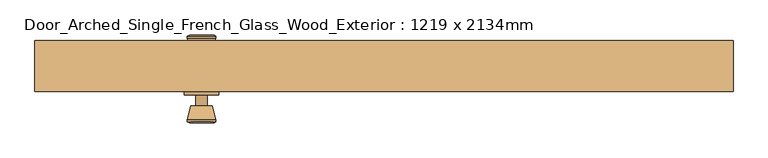
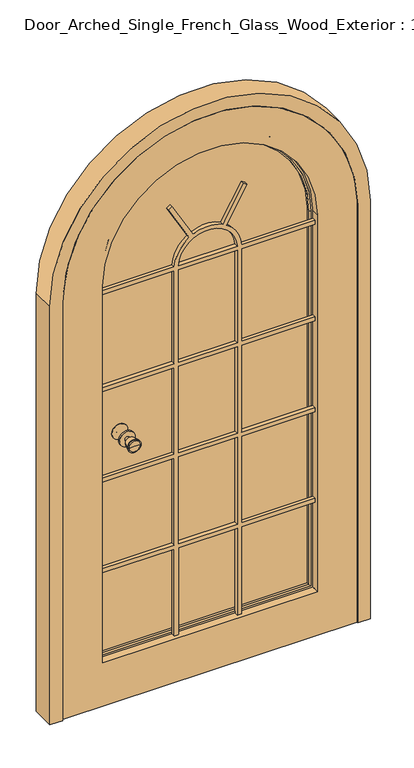
"""IFC4 building model written with IfcOpenShell, lengths in millimetres: door geometry, Door_Arched_Single_French_Glass_Wood_Exterior : 1219 x 2134mm."""

from ifc_helpers import new_model, si_unit, point, frame, frame_2d, origin, place, context, project, spatial, polyline, circle_curve, ellipse_curve, trimmed, segment, composite_curve, outline, extrude, source, transform, mapped, element, save
from ifc_brep_helpers import plane_surface, cylinder_surface, revolved_surface, advanced_brep


def door_arched_single_french_glass_wood_exterior_1219_x_2134mm_7a906126(model_context):
    return source(origin(), model_context, "Body", "SolidModel", [
        advanced_brep(
        [(-318.5, -5.7, 1050.0), (-308.5, -5.7, 1050.0), (-328.5, -5.7, 1050.0), (-298.0241324, -54.7, 1050.0), (-318.5, -54.7, 1050.0), (-338.9758676, -54.7, 1050.0), (-293.5, -52.8721319, 1050.0), (-343.5, -52.8721319, 1050.0), (-293.5, -49.4084537, 1050.0), (-343.5, -49.4084537, 1050.0), (-299.863764, -24.7, 1050.0), (-337.136236, -24.7, 1050.0), (-308.5, -24.7, 1050.0), (-328.5, -24.7, 1050.0)],
        [
            (0, 1),
            (1, 2, circle_curve(frame((-318.5, -5.7, 1050.0), z_axis=(0.0, 1.0, 0.0), x_axis=(-1.0, 0.0, 0.0)), 10.0)),
            (2, 0),
            (2, 1, circle_curve(frame((-318.5, -5.7, 1050.0), z_axis=(0.0, 1.0, 0.0), x_axis=(-1.0, 0.0, 0.0)), 10.0)),
            (3, 4),
            (4, 5),
            (5, 3, circle_curve(frame((-318.5, -54.7, 1050.0), z_axis=(0.0, -1.0, 0.0), x_axis=(-1.0, 0.0, 0.0)), 20.4758676)),
            (3, 5, circle_curve(frame((-318.5, -54.7, 1050.0), z_axis=(0.0, -1.0, 0.0), x_axis=(-1.0, 0.0, 0.0)), 20.4758676)),
            (6, 3),
            (5, 7),
            (7, 6, circle_curve(frame((-318.5, -52.8721319, 1050.0), z_axis=(0.0, -1.0, 0.0), x_axis=(-1.0, 0.0, 0.0)), 25.0)),
            (6, 7, circle_curve(frame((-318.5, -52.8721319, 1050.0), z_axis=(0.0, -1.0, 0.0), x_axis=(-1.0, 0.0, 0.0)), 25.0)),
            (8, 6),
            (7, 9),
            (9, 8, circle_curve(frame((-318.5, -49.4084537, 1050.0), z_axis=(0.0, -1.0, 0.0), x_axis=(-1.0, 0.0, 0.0)), 25.0)),
            (8, 9, circle_curve(frame((-318.5, -49.4084537, 1050.0), z_axis=(0.0, -1.0, 0.0), x_axis=(-1.0, 0.0, 0.0)), 25.0)),
            (10, 8),
            (9, 11),
            (11, 10, circle_curve(frame((-318.5, -24.7, 1050.0), z_axis=(0.0, -1.0, 0.0), x_axis=(-1.0, 0.0, 0.0)), 18.636236)),
            (10, 11, circle_curve(frame((-318.5, -24.7, 1050.0), z_axis=(0.0, -1.0, 0.0), x_axis=(-1.0, 0.0, 0.0)), 18.636236)),
            (12, 10),
            (11, 13),
            (13, 12, circle_curve(frame((-318.5, -24.7, 1050.0), z_axis=(0.0, -1.0, 0.0), x_axis=(-1.0, 0.0, 0.0)), 10.0)),
            (12, 13, circle_curve(frame((-318.5, -24.7, 1050.0), z_axis=(0.0, -1.0, 0.0), x_axis=(-1.0, 0.0, 0.0)), 10.0)),
            (1, 12),
            (13, 2),
        ],
        [
            plane_surface(frame((-318.5, -5.7, 1050.0), z_axis=(0.0, 1.0, 0.0), x_axis=(-1.0, 0.0, 0.0))),
            plane_surface(frame((-318.5, -54.7, 1050.0), z_axis=(0.0, -1.0, 0.0), x_axis=(-1.0, 0.0, 0.0))),
            revolved_surface(polyline([(-338.9758676, -54.7, 1050.0), (-343.5, -52.8721319, 1050.0)]), (-318.5, -5.7, 1050.0), (0.0, 1.0, 0.0)),
            cylinder_surface(frame((-318.5, -5.7, 1050.0), z_axis=(0.0, 1.0, 0.0), x_axis=(-1.0, 0.0, 0.0)), 25.0),
            revolved_surface(polyline([(-343.5, -49.4084537, 1050.0), (-337.136236, -24.7, 1050.0)]), (-318.5, -5.7, 1050.0), (0.0, 1.0, 0.0)),
            plane_surface(frame((-318.5, -24.7, 1050.0), z_axis=(0.0, 1.0, 0.0), x_axis=(-1.0, 0.0, 0.0))),
            cylinder_surface(frame((-318.5, -5.7, 1050.0), z_axis=(0.0, 1.0, 0.0), x_axis=(-1.0, 0.0, 0.0)), 10.0),
        ],
        [
            (0, [[1, 2, 3]]),
            (0, [[-3, 4, -1]]),
            (1, [[5, 6, 7]]),
            (1, [[-6, -5, 8]]),
            (2, [[9, -7, 10, 11]]),
            (2, [[-10, -8, -9, 12]]),
            (3, [[13, -11, 14, 15]]),
            (3, [[-14, -12, -13, 16]]),
            (4, [[17, -15, 18, 19]]),
            (4, [[-18, -16, -17, 20]]),
            (5, [[21, -19, 22, 23]]),
            (5, [[-22, -20, -21, 24]]),
            (6, [[25, -23, 26, -2]]),
            (6, [[-26, -24, -25, -4]]),
        ],
    ),
        extrude(outline(composite_curve([segment(trimmed(circle_curve(frame_2d((1050.0, -318.5)), 30.0), [point((1050.0, -348.5))], [point((1050.0, -288.5))], False, "CARTESIAN"), True, "CONTINUOUS"), segment(trimmed(circle_curve(frame_2d((1050.0, -318.5)), 30.0), [point((1050.0, -288.5))], [point((1050.0, -348.5))], False, "CARTESIAN"), True, "CONTINUOUS")], self_intersect=False)), frame((0.0, -5.7, 0.0), z_axis=(0.0, 1.0, 0.0), x_axis=(0.0, 0.0, 1.0)), (0.0, 0.0, 1.0), 6.0),
        advanced_brep(
        [(-318.5, 50.3, 1050.0), (-328.5, 50.3, 1050.0), (-308.5, 50.3, 1050.0), (-298.0241324, 99.3, 1050.0), (-338.9758676, 99.3, 1050.0), (-318.5, 99.3, 1050.0), (-293.5, 97.4721319, 1050.0), (-343.5, 97.4721319, 1050.0), (-293.5, 94.0084537, 1050.0), (-343.5, 94.0084537, 1050.0), (-299.863764, 69.3, 1050.0), (-337.136236, 69.3, 1050.0), (-308.5, 69.3, 1050.0), (-328.5, 69.3, 1050.0)],
        [
            (0, 1),
            (1, 2, circle_curve(frame((-318.5, 50.3, 1050.0), z_axis=(0.0, -1.0, 0.0), x_axis=(-1.0, 0.0, 0.0)), 10.0)),
            (2, 0),
            (2, 1, circle_curve(frame((-318.5, 50.3, 1050.0), z_axis=(0.0, -1.0, 0.0), x_axis=(-1.0, 0.0, 0.0)), 10.0)),
            (3, 4, circle_curve(frame((-318.5, 99.3, 1050.0), z_axis=(0.0, 1.0, 0.0), x_axis=(-1.0, 0.0, 0.0)), 20.4758676)),
            (4, 5),
            (5, 3),
            (4, 3, circle_curve(frame((-318.5, 99.3, 1050.0), z_axis=(0.0, 1.0, 0.0), x_axis=(-1.0, 0.0, 0.0)), 20.4758676)),
            (6, 7, circle_curve(frame((-318.5, 97.4721319, 1050.0), z_axis=(0.0, 1.0, 0.0), x_axis=(-1.0, 0.0, 0.0)), 25.0)),
            (7, 4),
            (3, 6),
            (7, 6, circle_curve(frame((-318.5, 97.4721319, 1050.0), z_axis=(0.0, 1.0, 0.0), x_axis=(-1.0, 0.0, 0.0)), 25.0)),
            (8, 9, circle_curve(frame((-318.5, 94.0084537, 1050.0), z_axis=(0.0, 1.0, 0.0), x_axis=(-1.0, 0.0, 0.0)), 25.0)),
            (9, 7),
            (6, 8),
            (9, 8, circle_curve(frame((-318.5, 94.0084537, 1050.0), z_axis=(0.0, 1.0, 0.0), x_axis=(-1.0, 0.0, 0.0)), 25.0)),
            (10, 11, circle_curve(frame((-318.5, 69.3, 1050.0), z_axis=(0.0, 1.0, 0.0), x_axis=(-1.0, 0.0, 0.0)), 18.636236)),
            (11, 9),
            (8, 10),
            (11, 10, circle_curve(frame((-318.5, 69.3, 1050.0), z_axis=(0.0, 1.0, 0.0), x_axis=(-1.0, 0.0, 0.0)), 18.636236)),
            (12, 13, circle_curve(frame((-318.5, 69.3, 1050.0), z_axis=(0.0, 1.0, 0.0), x_axis=(-1.0, 0.0, 0.0)), 10.0)),
            (13, 11),
            (10, 12),
            (13, 12, circle_curve(frame((-318.5, 69.3, 1050.0), z_axis=(0.0, 1.0, 0.0), x_axis=(-1.0, 0.0, 0.0)), 10.0)),
            (1, 13),
            (12, 2),
        ],
        [
            plane_surface(frame((-318.5, 50.3, 1050.0), z_axis=(0.0, -1.0, 0.0), x_axis=(-1.0, 0.0, 0.0))),
            plane_surface(frame((-318.5, 99.3, 1050.0), z_axis=(0.0, 1.0, 0.0), x_axis=(-1.0, 0.0, 0.0))),
            revolved_surface(polyline([(-338.9758676, 99.3, 1050.0), (-343.5, 97.4721319, 1050.0)]), (-318.5, 50.3, 1050.0), (0.0, -1.0, 0.0)),
            cylinder_surface(frame((-318.5, 50.3, 1050.0), z_axis=(0.0, -1.0, 0.0), x_axis=(-1.0, 0.0, 0.0)), 25.0),
            revolved_surface(polyline([(-343.5, 94.0084537, 1050.0), (-337.136236, 69.3, 1050.0)]), (-318.5, 50.3, 1050.0), (0.0, -1.0, 0.0)),
            plane_surface(frame((-318.5, 69.3, 1050.0), z_axis=(0.0, -1.0, 0.0), x_axis=(-1.0, 0.0, 0.0))),
            cylinder_surface(frame((-318.5, 50.3, 1050.0), z_axis=(0.0, -1.0, 0.0), x_axis=(-1.0, 0.0, 0.0)), 10.0),
        ],
        [
            (0, [[1, 2, 3]]),
            (0, [[-3, 4, -1]]),
            (1, [[5, 6, 7]]),
            (1, [[8, -7, -6]]),
            (2, [[9, 10, -5, 11]]),
            (2, [[12, -11, -8, -10]]),
            (3, [[13, 14, -9, 15]]),
            (3, [[16, -15, -12, -14]]),
            (4, [[17, 18, -13, 19]]),
            (4, [[20, -19, -16, -18]]),
            (5, [[21, 22, -17, 23]]),
            (5, [[24, -23, -20, -22]]),
            (6, [[-2, 25, -21, 26]]),
            (6, [[-4, -26, -24, -25]]),
        ],
    ),
        extrude(outline(composite_curve([segment(trimmed(circle_curve(frame_2d((1050.0, -318.5)), 30.0), [point((1050.0, -348.5))], [point((1050.0, -288.5))], False, "CARTESIAN"), True, "CONTINUOUS"), segment(trimmed(circle_curve(frame_2d((1050.0, -318.5)), 30.0), [point((1050.0, -288.5))], [point((1050.0, -348.5))], False, "CARTESIAN"), True, "CONTINUOUS")], self_intersect=False)), frame((0.0, 44.3, 0.0), z_axis=(0.0, 1.0, 0.0), x_axis=(0.0, 0.0, 1.0)), (0.0, 0.0, 1.0), 6.0),
        advanced_brep(
        [(539.1, 89.3, 0.0), (609.6, 89.3, 0.0), (609.6, 0.3, 0.0), (561.1, 0.3, 0.0), (561.1, 47.3, 0.0), (539.1, 47.3, 0.0), (539.1, 89.3, 1678.6), (-539.1, 89.3, 1678.6), (-539.1, 89.3, 0.0), (-609.6, 89.3, 0.0), (-609.6, 89.3, 1678.6), (609.6, 89.3, 1678.6), (609.6, 0.3, 1678.6), (-609.6, 0.3, 1678.6), (-609.6, 0.3, 0.0), (-561.1, 0.3, 0.0), (-561.1, 0.3, 1678.6), (561.1, 0.3, 1678.6), (561.1, 47.3, 1678.6), (-561.1, 47.3, 1678.6), (-561.1, 47.3, 0.0), (-539.1, 47.3, 0.0), (-539.1, 47.3, 1678.6), (539.1, 47.3, 1678.6)],
        [
            (0, 1),
            (1, 2),
            (2, 3),
            (3, 4),
            (4, 5),
            (5, 0),
            (0, 6),
            (6, 7, circle_curve(frame((0.0, 89.3, 1678.6), z_axis=(0.0, -1.0, 0.0), x_axis=(1.0, 0.0, 0.0)), 539.1)),
            (7, 8),
            (8, 9),
            (9, 10),
            (10, 11, circle_curve(frame((0.0, 89.3, 1678.6), z_axis=(0.0, 1.0, 0.0), x_axis=(1.0, 0.0, 0.0)), 609.6)),
            (11, 1),
            (11, 12),
            (12, 2),
            (12, 13, circle_curve(frame((0.0, 0.3, 1678.6), z_axis=(0.0, -1.0, 0.0), x_axis=(1.0, 0.0, 0.0)), 609.6)),
            (13, 14),
            (14, 15),
            (15, 16),
            (16, 17, circle_curve(frame((0.0, 0.3, 1678.6), z_axis=(0.0, 1.0, 0.0), x_axis=(1.0, 0.0, 0.0)), 561.1)),
            (17, 3),
            (17, 18),
            (18, 4),
            (18, 19, circle_curve(frame((0.0, 47.3, 1678.6), z_axis=(0.0, -1.0, 0.0), x_axis=(1.0, 0.0, 0.0)), 561.1)),
            (19, 20),
            (20, 21),
            (21, 22),
            (22, 23, circle_curve(frame((0.0, 47.3, 1678.6), z_axis=(0.0, 1.0, 0.0), x_axis=(1.0, 0.0, 0.0)), 539.1)),
            (23, 5),
            (23, 6),
            (7, 22),
            (21, 8),
            (20, 15),
            (14, 9),
            (13, 10),
            (19, 16),
        ],
        [
            plane_surface(frame((603.1, -9.1123976, 0.0), z_axis=(0.0, 0.0, -1.0), x_axis=(1.0, 0.0, 0.0))),
            plane_surface(frame((539.1, 89.3, 0.0), z_axis=(0.0, 1.0, 0.0), x_axis=(0.0, 0.0, 1.0))),
            plane_surface(frame((609.6, 89.3, 0.0), z_axis=(1.0, 0.0, 0.0), x_axis=(0.0, 0.0, 1.0))),
            plane_surface(frame((609.6, 0.3, 0.0), z_axis=(0.0, -1.0, 0.0), x_axis=(0.0, 0.0, 1.0))),
            plane_surface(frame((561.1, 0.3, 0.0), z_axis=(-1.0, 0.0, 0.0), x_axis=(0.0, 0.0, 1.0))),
            plane_surface(frame((561.1, 47.3, 0.0), z_axis=(0.0, -1.0, 0.0), x_axis=(0.0, 0.0, 1.0))),
            plane_surface(frame((539.1, 47.3, 0.0), z_axis=(-1.0, 0.0, 0.0), x_axis=(0.0, 0.0, 1.0))),
            plane_surface(frame((-539.1, 47.3, 1678.6), z_axis=(1.0, 0.0, 0.0), x_axis=(0.0, 0.0, -1.0))),
            plane_surface(frame((-603.1, -9.1123976, 0.0), z_axis=(0.0, 0.0, -1.0), x_axis=(-1.0, 0.0, 0.0))),
            plane_surface(frame((-609.6, 89.3, 1678.6), z_axis=(-1.0, 0.0, 0.0), x_axis=(0.0, 0.0, -1.0))),
            plane_surface(frame((-561.1, 0.3, 1678.6), z_axis=(1.0, 0.0, 0.0), x_axis=(0.0, 0.0, -1.0))),
            cylinder_surface(frame((0.0, 89.3, 1678.6), z_axis=(0.0, -1.0, 0.0), x_axis=(1.0, 0.0, 0.0)), 609.6),
            revolved_surface(polyline([(561.1, 0.29999999999999716, 1678.6), (561.1, 47.3, 1678.6)]), (0.0, 89.3, 1678.6), (0.0, -1.0, 0.0)),
            revolved_surface(polyline([(539.1, 47.3, 1678.6), (539.1, 89.3, 1678.6)]), (0.0, 89.3, 1678.6), (0.0, -1.0, 0.0)),
        ],
        [
            (0, [[1, 2, 3, 4, 5, 6]]),
            (1, [[-1, 7, 8, 9, 10, 11, 12, 13]]),
            (2, [[-2, -13, 14, 15]]),
            (3, [[-3, -15, 16, 17, 18, 19, 20, 21]]),
            (4, [[-4, -21, 22, 23]]),
            (5, [[-5, -23, 24, 25, 26, 27, 28, 29]]),
            (6, [[-6, -29, 30, -7]]),
            (7, [[31, -27, 32, -9]]),
            (8, [[-32, -26, 33, -18, 34, -10]]),
            (9, [[35, -11, -34, -17]]),
            (10, [[36, -19, -33, -25]]),
            (11, [[-16, -14, -12, -35]]),
            (12, [[-24, -22, -20, -36]]),
            (13, [[-8, -30, -28, -31]]),
        ],
    ),
        extrude(outline(composite_curve([segment(trimmed(circle_curve(frame_2d((1692.1, 0.0)), 253.5), [point((1896.740356, 149.6147543))], [point((1905.7961472, 136.3679092))], False, "CARTESIAN"), True, "CONTINUOUS"), segment(polyline([(1905.7961472, 136.3679092), (1768.2345335, 56.9466745)]), True, "CONTINUOUS"), segment(trimmed(circle_curve(frame_2d((1653.6, 0.0)), 128.0), [point((1768.2345335, 56.9466745))], [point((1768.2345335, -56.9466745))], False, "CARTESIAN"), True, "CONTINUOUS"), segment(polyline([(1768.2345335, -56.9466745), (1905.7961472, -136.3679092)]), True, "CONTINUOUS"), segment(trimmed(circle_curve(frame_2d((1692.1, 0.0)), 253.5), [point((1905.7961472, -136.3679092))], [point((1896.740356, -149.6147543))], False, "CARTESIAN"), True, "CONTINUOUS"), segment(polyline([(1896.740356, -149.6147543), (1760.2345335, -70.8030809)]), True, "CONTINUOUS"), segment(trimmed(circle_curve(frame_2d((1653.6, 0.0)), 128.0), [point((1760.2345335, -70.8030809))], [point((1661.6, -127.7497554))], False, "CARTESIAN"), True, "CONTINUOUS"), segment(polyline([(1661.6, -127.7497554), (1661.6, -408.1), (1645.6, -408.1), (1645.6, -128.0), (1273.5, -128.0), (1273.5, -408.1), (1257.5, -408.1), (1257.5, -128.0), (909.0, -128.0), (909.0, -408.1), (893.0, -408.1), (893.0, -128.0), (544.5, -128.0), (544.5, -408.1), (528.5, -408.1), (528.5, -128.0), (179.0, -128.0), (179.0, -112.0), (528.5, -112.0), (528.5, 112.0), (179.0, 112.0), (179.0, 128.0), (528.5, 128.0), (528.5, 408.1), (544.5, 408.1), (544.5, 128.0), (893.0, 128.0), (893.0, 408.1), (909.0, 408.1), (909.0, 128.0), (1257.5, 128.0), (1257.5, 408.1), (1273.5, 408.1), (1273.5, 128.0), (1645.6, 128.0), (1645.6, 408.1), (1661.6, 408.1), (1661.6, 127.7497554)]), True, "CONTINUOUS"), segment(trimmed(circle_curve(frame_2d((1653.6, 0.0)), 128.0), [point((1661.6, 127.7497554))], [point((1760.2345335, 70.8030809))], False, "CARTESIAN"), True, "CONTINUOUS"), segment(polyline([(1760.2345335, 70.8030809), (1896.740356, 149.6147543)]), True, "CONTINUOUS")], self_intersect=False), holes=[polyline([(893.0, -112.0), (893.0, 112.0), (544.5, 112.0), (544.5, -112.0), (893.0, -112.0)]), polyline([(1257.5, 112.0), (909.0, 112.0), (909.0, -112.0), (1257.5, -112.0), (1257.5, 112.0)]), composite_curve([segment(trimmed(circle_curve(frame_2d((1653.6, 0.0)), 112.0), [point((1661.6, -111.7139204))], [point((1661.6, 111.7139204))], True, "CARTESIAN"), True, "CONTINUOUS"), segment(polyline([(1661.6, 111.7139204), (1661.6, -111.7139204)]), True, "CONTINUOUS")], self_intersect=False), polyline([(1645.6, -112.0), (1645.6, 112.0), (1273.5, 112.0), (1273.5, -112.0), (1645.6, -112.0)])]), frame((0.0, 15.1515468, 0.0), z_axis=(0.0, 1.0, 0.0), x_axis=(0.0, 0.0, 1.0)), (0.0, 0.0, 1.0), 14.5359085),
        extrude(outline(composite_curve([segment(polyline([(4.0, 558.1), (1727.8950302, 558.1)]), True, "CONTINUOUS"), segment(trimmed(circle_curve(frame_2d((1678.6, 0.0)), 560.2727996), [point((1727.8950302, 558.1))], [point((1715.9714663, -559.0250294))], False, "CARTESIAN"), True, "CONTINUOUS"), segment(polyline([(1715.9714663, -559.0250294), (4.0, -559.0250294), (4.0, 558.1)]), True, "CONTINUOUS")], self_intersect=False), holes=[composite_curve([segment(polyline([(179.0, -408.1), (1692.1, -408.1)]), True, "CONTINUOUS"), segment(trimmed(circle_curve(frame_2d((1692.1, 0.0)), 408.1), [point((1692.1, -408.1))], [point((1692.1, 408.1))], True, "CARTESIAN"), True, "CONTINUOUS"), segment(polyline([(1692.1, 408.1), (179.0, 408.1), (179.0, -408.1)]), True, "CONTINUOUS")], self_intersect=False)]), frame((0.0, 0.3, 0.0), z_axis=(0.0, 1.0, 0.0), x_axis=(0.0, 0.0, 1.0)), (0.0, 0.0, 1.0), 44.0),
        extrude(outline(composite_curve([segment(polyline([(179.0, -408.1), (179.0, 408.1), (1692.1, 408.1)]), True, "CONTINUOUS"), segment(trimmed(circle_curve(frame_2d((1692.1, 0.0)), 408.1), [point((1692.1, 408.1))], [point((1692.1, -408.1))], False, "CARTESIAN"), True, "CONTINUOUS"), segment(polyline([(1692.1, -408.1), (179.0, -408.1)]), True, "CONTINUOUS")], self_intersect=False)), frame((0.0, 46.0, 0.0), z_axis=(0.0, 1.0, 0.0), x_axis=(0.0, 0.0, 1.0)), (0.0, 0.0, 1.0), 24.0),
        advanced_brep(
        [(-416.1, 84.0, 171.0), (-416.1, 80.0, 171.0), (-416.1, 80.0, 1692.1), (-416.1, 84.0, 1692.1), (-414.1, 86.0, 173.0), (-414.1, 86.0, 1692.1), (-396.1, 81.0, 191.0), (-401.1, 86.0, 186.0), (-401.1, 86.0, 1692.1), (-396.1, 81.0, 1692.1), (-396.1, 70.0, 191.0), (-396.1, 70.0, 1692.1), (-408.1, 80.0, 179.0), (-408.1, 70.0, 179.0), (-408.1, 70.0, 1692.1), (-408.1, 80.0, 1692.1), (416.1, 84.0, 1692.1), (416.1, 80.0, 1692.1), (414.1, 86.0, 1692.1), (414.1, 86.0, 173.0), (401.1, 86.0, 1692.1), (401.1, 86.0, 186.0), (396.1, 81.0, 1692.1), (396.1, 70.0, 1692.1), (408.1, 70.0, 1692.1), (408.1, 70.0, 179.0), (396.1, 70.0, 191.0), (408.1, 80.0, 1692.1), (416.1, 80.0, 171.0), (408.1, 80.0, 179.0), (416.1, 84.0, 171.0), (396.1, 81.0, 191.0)],
        [
            (0, 1),
            (1, 2),
            (2, 3),
            (3, 0),
            (4, 0, ellipse_curve(frame((-414.1, 84.0, 173.0), z_axis=(-0.7071067811865475, 0.0, 0.7071067811865475), x_axis=(-0.7071067811865474, 0.0, -0.7071067811865476)), 2.8284271, 2.0)),
            (3, 5, circle_curve(frame((-414.1, 84.0, 1692.1), z_axis=(0.0, 0.0, -1.0), x_axis=(-1.0, 0.0, 0.0)), 2.0)),
            (5, 4),
            (6, 7, ellipse_curve(frame((-401.1, 81.0, 186.0), z_axis=(-0.7071067811865475, 0.0, 0.7071067811865475), x_axis=(-0.7071067811865474, 0.0, -0.7071067811865476)), 7.0710678, 5.0)),
            (7, 8),
            (8, 9, circle_curve(frame((-401.1, 81.0, 1692.1), z_axis=(0.0, 0.0, -1.0), x_axis=(-1.0, 0.0, 0.0)), 5.0)),
            (9, 6),
            (10, 6),
            (9, 11),
            (11, 10),
            (12, 13),
            (13, 14),
            (14, 15),
            (15, 12),
            (16, 3, circle_curve(frame((0.0, 84.0, 1692.1), z_axis=(0.0, -1.0, 0.0), x_axis=(-1.0, 0.0, 0.0)), 416.1)),
            (2, 17, circle_curve(frame((0.0, 80.0, 1692.1), z_axis=(0.0, 1.0, 0.0), x_axis=(-1.0, 0.0, 0.0)), 416.1)),
            (17, 16),
            (18, 5, circle_curve(frame((0.0, 86.0, 1692.1), z_axis=(0.0, -1.0, 0.0), x_axis=(-1.0, 0.0, 0.0)), 414.1)),
            (16, 18, circle_curve(frame((414.1, 84.0, 1692.1), z_axis=(0.0, 0.0, 1.0), x_axis=(1.0, 0.0, 0.0)), 2.0)),
            (18, 19),
            (19, 4),
            (20, 8, circle_curve(frame((0.0, 86.0, 1692.1), z_axis=(0.0, -1.0, 0.0), x_axis=(-1.0, 0.0, 0.0)), 401.1)),
            (7, 21),
            (21, 20),
            (22, 9, circle_curve(frame((0.0, 81.0, 1692.1), z_axis=(0.0, -1.0, 0.0), x_axis=(-1.0, 0.0, 0.0)), 396.1)),
            (20, 22, circle_curve(frame((401.1, 81.0, 1692.1), z_axis=(0.0, 0.0, 1.0), x_axis=(1.0, 0.0, 0.0)), 5.0)),
            (23, 11, circle_curve(frame((0.0, 70.0, 1692.1), z_axis=(0.0, -1.0, 0.0), x_axis=(-1.0, 0.0, 0.0)), 396.1)),
            (22, 23),
            (24, 14, circle_curve(frame((0.0, 70.0, 1692.1), z_axis=(0.0, -1.0, 0.0), x_axis=(-1.0, 0.0, 0.0)), 408.1)),
            (13, 25),
            (25, 24),
            (23, 26),
            (26, 10),
            (27, 15, circle_curve(frame((0.0, 80.0, 1692.1), z_axis=(0.0, -1.0, 0.0), x_axis=(-1.0, 0.0, 0.0)), 408.1)),
            (24, 27),
            (1, 28),
            (28, 17),
            (27, 29),
            (29, 12),
            (28, 30),
            (30, 16),
            (30, 19, ellipse_curve(frame((414.1, 84.0, 173.0), z_axis=(0.7071067811865475, 0.0, 0.7071067811865475), x_axis=(-0.7071067811865474, 0.0, 0.7071067811865476)), 2.8284271, 2.0)),
            (21, 31, ellipse_curve(frame((401.1, 81.0, 186.0), z_axis=(0.7071067811865475, 0.0, 0.7071067811865475), x_axis=(-0.7071067811865474, 0.0, 0.7071067811865476)), 7.0710678, 5.0)),
            (31, 22),
            (31, 26),
            (25, 29),
            (0, 30),
            (6, 31),
        ],
        [
            plane_surface(frame((-416.1, 80.0, 171.0), z_axis=(-1.0, 0.0, 0.0), x_axis=(0.0, 0.0, 1.0))),
            cylinder_surface(frame((-414.1, 84.0, 179.0), z_axis=(0.0, 0.0, -1.0), x_axis=(-1.0, 0.0, 0.0)), 2.0),
            cylinder_surface(frame((-401.1, 81.0, 179.0), z_axis=(0.0, 0.0, -1.0), x_axis=(-1.0, 0.0, 0.0)), 5.0),
            plane_surface(frame((-396.1, 81.0, 191.0), z_axis=(1.0, 0.0, 0.0), x_axis=(0.0, 0.0, 1.0))),
            plane_surface(frame((-408.1, 70.0, 179.0), z_axis=(-1.0, 0.0, 0.0), x_axis=(0.0, 0.0, 1.0))),
            cylinder_surface(frame((0.0, 80.0, 1692.1), z_axis=(0.0, 1.0, 0.0), x_axis=(-1.0, 0.0, 0.0)), 416.1),
            revolved_surface(trimmed(ellipse_curve(frame((-414.1, 84.0, 1692.1), z_axis=(0.0, 0.0, -1.0), x_axis=(-1.0, 0.0, 0.0)), 2.0, 2.0), [point((-416.1, 84.0, 1692.1))], [point((-414.1, 86.0, 1692.1))], True, "CARTESIAN"), (0.0, 80.0, 1692.1), (0.0, 1.0, 0.0)),
            plane_surface(frame((0.0, 86.0, 1692.1), z_axis=(0.0, 1.0, 0.0), x_axis=(-1.0, 0.0, 0.0))),
            revolved_surface(trimmed(ellipse_curve(frame((-401.1, 81.0, 1692.1), z_axis=(0.0, 0.0, -1.0), x_axis=(-1.0, 0.0, 0.0)), 5.0, 5.0), [point((-401.1, 86.0, 1692.1))], [point((-396.1, 81.0, 1692.1))], True, "CARTESIAN"), (0.0, 80.0, 1692.1), (0.0, 1.0, 0.0)),
            revolved_surface(polyline([(-396.1, 81.0, 1692.1), (-396.1, 70.0, 1692.1)]), (0.0, 80.0, 1692.1), (0.0, 1.0, 0.0)),
            plane_surface(frame((0.0, 70.0, 1692.1), z_axis=(0.0, -1.0, 0.0), x_axis=(-1.0, 0.0, 0.0))),
            cylinder_surface(frame((0.0, 80.0, 1692.1), z_axis=(0.0, 1.0, 0.0), x_axis=(-1.0, 0.0, 0.0)), 408.1),
            plane_surface(frame((0.0, 80.0, 1692.1), z_axis=(0.0, -1.0, 0.0), x_axis=(-1.0, 0.0, 0.0))),
            plane_surface(frame((416.1, 80.0, 1692.1), z_axis=(1.0, 0.0, 0.0), x_axis=(0.0, 0.0, -1.0))),
            cylinder_surface(frame((414.1, 84.0, 1692.1), z_axis=(0.0, 0.0, 1.0), x_axis=(1.0, 0.0, 0.0)), 2.0),
            cylinder_surface(frame((401.1, 81.0, 1692.1), z_axis=(0.0, 0.0, 1.0), x_axis=(1.0, 0.0, 0.0)), 5.0),
            plane_surface(frame((396.1, 81.0, 1692.1), z_axis=(-1.0, 0.0, 0.0), x_axis=(0.0, 0.0, -1.0))),
            plane_surface(frame((408.1, 70.0, 1692.1), z_axis=(1.0, 0.0, 0.0), x_axis=(0.0, 0.0, -1.0))),
            plane_surface(frame((416.1, 80.0, 171.0), z_axis=(0.0, 0.0, -1.0), x_axis=(-1.0, 0.0, 0.0))),
            cylinder_surface(frame((408.1, 84.0, 173.0), z_axis=(1.0, 0.0, 0.0), x_axis=(0.0, 0.0, -1.0)), 2.0),
            cylinder_surface(frame((408.1, 81.0, 186.0), z_axis=(1.0, 0.0, 0.0), x_axis=(0.0, 0.0, -1.0)), 5.0),
            plane_surface(frame((396.1, 81.0, 191.0), z_axis=(0.0, 0.0, 1.0), x_axis=(-1.0, 0.0, 0.0))),
            plane_surface(frame((408.1, 70.0, 179.0), z_axis=(0.0, 0.0, -1.0), x_axis=(-1.0, 0.0, 0.0))),
        ],
        [
            (0, [[1, 2, 3, 4]]),
            (1, [[5, -4, 6, 7]]),
            (2, [[8, 9, 10, 11]]),
            (3, [[12, -11, 13, 14]]),
            (4, [[15, 16, 17, 18]]),
            (5, [[19, -3, 20, 21]]),
            (6, [[22, -6, -19, 23]]),
            (7, [[24, 25, -7, -22], [26, -9, 27, 28]]),
            (8, [[29, -10, -26, 30]]),
            (9, [[31, -13, -29, 32]]),
            (10, [[33, -16, 34, 35], [36, 37, -14, -31]]),
            (11, [[38, -17, -33, 39]]),
            (12, [[-20, -2, 40, 41], [42, 43, -18, -38]]),
            (13, [[-21, -41, 44, 45]]),
            (14, [[-23, -45, 46, -24]]),
            (15, [[-30, -28, 47, 48]]),
            (16, [[-32, -48, 49, -36]]),
            (17, [[-39, -35, 50, -42]]),
            (18, [[-44, -40, -1, 51]]),
            (19, [[-46, -51, -5, -25]]),
            (20, [[-47, -27, -8, 52]]),
            (21, [[-49, -52, -12, -37]]),
            (22, [[-50, -34, -15, -43]]),
        ],
    ),
        advanced_brep(
        [(416.1, 32.0, 171.0), (416.1, 36.0, 171.0), (416.1, 36.0, 1692.1), (416.1, 32.0, 1692.1), (414.1, 30.0, 173.0), (414.1, 30.0, 1692.1), (396.1, 35.0, 191.0), (401.1, 30.0, 186.0), (401.1, 30.0, 1692.1), (396.1, 35.0, 1692.1), (396.1, 46.0, 191.0), (396.1, 46.0, 1692.1), (408.1, 36.0, 179.0), (408.1, 46.0, 179.0), (408.1, 46.0, 1692.1), (408.1, 36.0, 1692.1), (-416.1, 32.0, 1692.1), (-416.1, 36.0, 1692.1), (-414.1, 30.0, 1692.1), (-414.1, 30.0, 173.0), (-401.1, 30.0, 1692.1), (-401.1, 30.0, 186.0), (-396.1, 35.0, 1692.1), (-396.1, 46.0, 1692.1), (-408.1, 46.0, 1692.1), (-408.1, 46.0, 179.0), (-396.1, 46.0, 191.0), (-408.1, 36.0, 1692.1), (-416.1, 36.0, 171.0), (-408.1, 36.0, 179.0), (-416.1, 32.0, 171.0), (-396.1, 35.0, 191.0)],
        [
            (0, 1),
            (1, 2),
            (2, 3),
            (3, 0),
            (4, 0, ellipse_curve(frame((414.1, 32.0, 173.0), z_axis=(0.7071067811865475, 0.0, 0.7071067811865475), x_axis=(0.7071067811865474, 0.0, -0.7071067811865476)), 2.8284271, 2.0)),
            (3, 5, circle_curve(frame((414.1, 32.0, 1692.1), z_axis=(0.0, 0.0, -1.0), x_axis=(1.0, 0.0, 0.0)), 2.0)),
            (5, 4),
            (6, 7, ellipse_curve(frame((401.1, 35.0, 186.0), z_axis=(0.7071067811865475, 0.0, 0.7071067811865475), x_axis=(0.7071067811865474, 0.0, -0.7071067811865476)), 7.0710678, 5.0)),
            (7, 8),
            (8, 9, circle_curve(frame((401.1, 35.0, 1692.1), z_axis=(0.0, 0.0, -1.0), x_axis=(1.0, 0.0, 0.0)), 5.0)),
            (9, 6),
            (10, 6),
            (9, 11),
            (11, 10),
            (12, 13),
            (13, 14),
            (14, 15),
            (15, 12),
            (16, 3, circle_curve(frame((0.0, 32.0, 1692.1), z_axis=(0.0, 1.0, 0.0), x_axis=(1.0, 0.0, 0.0)), 416.1)),
            (2, 17, circle_curve(frame((0.0, 36.0, 1692.1), z_axis=(0.0, -1.0, 0.0), x_axis=(1.0, 0.0, 0.0)), 416.1)),
            (17, 16),
            (18, 5, circle_curve(frame((0.0, 30.0, 1692.1), z_axis=(0.0, 1.0, 0.0), x_axis=(1.0, 0.0, 0.0)), 414.1)),
            (16, 18, circle_curve(frame((-414.1, 32.0, 1692.1), z_axis=(0.0, 0.0, 1.0), x_axis=(-1.0, 0.0, 0.0)), 2.0)),
            (18, 19),
            (19, 4),
            (20, 8, circle_curve(frame((0.0, 30.0, 1692.1), z_axis=(0.0, 1.0, 0.0), x_axis=(1.0, 0.0, 0.0)), 401.1)),
            (7, 21),
            (21, 20),
            (22, 9, circle_curve(frame((0.0, 35.0, 1692.1), z_axis=(0.0, 1.0, 0.0), x_axis=(1.0, 0.0, 0.0)), 396.1)),
            (20, 22, circle_curve(frame((-401.1, 35.0, 1692.1), z_axis=(0.0, 0.0, 1.0), x_axis=(-1.0, 0.0, 0.0)), 5.0)),
            (23, 11, circle_curve(frame((0.0, 46.0, 1692.1), z_axis=(0.0, 1.0, 0.0), x_axis=(1.0, 0.0, 0.0)), 396.1)),
            (22, 23),
            (24, 14, circle_curve(frame((0.0, 46.0, 1692.1), z_axis=(0.0, 1.0, 0.0), x_axis=(1.0, 0.0, 0.0)), 408.1)),
            (13, 25),
            (25, 24),
            (23, 26),
            (26, 10),
            (27, 15, circle_curve(frame((0.0, 36.0, 1692.1), z_axis=(0.0, 1.0, 0.0), x_axis=(1.0, 0.0, 0.0)), 408.1)),
            (24, 27),
            (1, 28),
            (28, 17),
            (27, 29),
            (29, 12),
            (28, 30),
            (30, 16),
            (30, 19, ellipse_curve(frame((-414.1, 32.0, 173.0), z_axis=(-0.7071067811865475, 0.0, 0.7071067811865475), x_axis=(0.7071067811865474, 0.0, 0.7071067811865476)), 2.8284271, 2.0)),
            (21, 31, ellipse_curve(frame((-401.1, 35.0, 186.0), z_axis=(-0.7071067811865475, 0.0, 0.7071067811865475), x_axis=(0.7071067811865474, 0.0, 0.7071067811865476)), 7.0710678, 5.0)),
            (31, 22),
            (31, 26),
            (25, 29),
            (0, 30),
            (6, 31),
        ],
        [
            plane_surface(frame((416.1, 36.0, 171.0), z_axis=(1.0, 0.0, 0.0), x_axis=(0.0, 0.0, 1.0))),
            cylinder_surface(frame((414.1, 32.0, 179.0), z_axis=(0.0, 0.0, -1.0), x_axis=(1.0, 0.0, 0.0)), 2.0),
            cylinder_surface(frame((401.1, 35.0, 179.0), z_axis=(0.0, 0.0, -1.0), x_axis=(1.0, 0.0, 0.0)), 5.0),
            plane_surface(frame((396.1, 35.0, 191.0), z_axis=(-1.0, 0.0, 0.0), x_axis=(0.0, 0.0, 1.0))),
            plane_surface(frame((408.1, 46.0, 179.0), z_axis=(1.0, 0.0, 0.0), x_axis=(0.0, 0.0, 1.0))),
            cylinder_surface(frame((0.0, 36.0, 1692.1), z_axis=(0.0, -1.0, 0.0), x_axis=(1.0, 0.0, 0.0)), 416.1),
            revolved_surface(trimmed(ellipse_curve(frame((414.1, 32.0, 1692.1), z_axis=(0.0, 0.0, -1.0), x_axis=(1.0, 0.0, 0.0)), 2.0, 2.0), [point((416.1, 32.0, 1692.1))], [point((414.1, 30.0, 1692.1))], True, "CARTESIAN"), (0.0, 36.0, 1692.1), (0.0, -1.0, 0.0)),
            plane_surface(frame((0.0, 30.0, 1692.1), z_axis=(0.0, -1.0, 0.0), x_axis=(1.0, 0.0, 0.0))),
            revolved_surface(trimmed(ellipse_curve(frame((401.1, 35.0, 1692.1), z_axis=(0.0, 0.0, -1.0), x_axis=(1.0, 0.0, 0.0)), 5.0, 5.0), [point((401.1, 30.0, 1692.1))], [point((396.1, 35.0, 1692.1))], True, "CARTESIAN"), (0.0, 36.0, 1692.1), (0.0, -1.0, 0.0)),
            revolved_surface(polyline([(396.1, 35.0, 1692.1), (396.1, 46.0, 1692.1)]), (0.0, 36.0, 1692.1), (0.0, -1.0, 0.0)),
            plane_surface(frame((0.0, 46.0, 1692.1), z_axis=(0.0, 1.0, 0.0), x_axis=(1.0, 0.0, 0.0))),
            cylinder_surface(frame((0.0, 36.0, 1692.1), z_axis=(0.0, -1.0, 0.0), x_axis=(1.0, 0.0, 0.0)), 408.1),
            plane_surface(frame((0.0, 36.0, 1692.1), z_axis=(0.0, 1.0, 0.0), x_axis=(1.0, 0.0, 0.0))),
            plane_surface(frame((-416.1, 36.0, 1692.1), z_axis=(-1.0, 0.0, 0.0), x_axis=(0.0, 0.0, -1.0))),
            cylinder_surface(frame((-414.1, 32.0, 1692.1), z_axis=(0.0, 0.0, 1.0), x_axis=(-1.0, 0.0, 0.0)), 2.0),
            cylinder_surface(frame((-401.1, 35.0, 1692.1), z_axis=(0.0, 0.0, 1.0), x_axis=(-1.0, 0.0, 0.0)), 5.0),
            plane_surface(frame((-396.1, 35.0, 1692.1), z_axis=(1.0, 0.0, 0.0), x_axis=(0.0, 0.0, -1.0))),
            plane_surface(frame((-408.1, 46.0, 1692.1), z_axis=(-1.0, 0.0, 0.0), x_axis=(0.0, 0.0, -1.0))),
            plane_surface(frame((-416.1, 36.0, 171.0), z_axis=(0.0, 0.0, -1.0), x_axis=(1.0, 0.0, 0.0))),
            cylinder_surface(frame((-408.1, 32.0, 173.0), z_axis=(-1.0, 0.0, 0.0), x_axis=(0.0, 0.0, -1.0)), 2.0),
            cylinder_surface(frame((-408.1, 35.0, 186.0), z_axis=(-1.0, 0.0, 0.0), x_axis=(0.0, 0.0, -1.0)), 5.0),
            plane_surface(frame((-396.1, 35.0, 191.0), z_axis=(0.0, 0.0, 1.0), x_axis=(1.0, 0.0, 0.0))),
            plane_surface(frame((-408.1, 46.0, 179.0), z_axis=(0.0, 0.0, -1.0), x_axis=(1.0, 0.0, 0.0))),
        ],
        [
            (0, [[1, 2, 3, 4]]),
            (1, [[5, -4, 6, 7]]),
            (2, [[8, 9, 10, 11]]),
            (3, [[12, -11, 13, 14]]),
            (4, [[15, 16, 17, 18]]),
            (5, [[19, -3, 20, 21]]),
            (6, [[22, -6, -19, 23]]),
            (7, [[24, 25, -7, -22], [26, -9, 27, 28]]),
            (8, [[29, -10, -26, 30]]),
            (9, [[31, -13, -29, 32]]),
            (10, [[33, -16, 34, 35], [36, 37, -14, -31]]),
            (11, [[38, -17, -33, 39]]),
            (12, [[-20, -2, 40, 41], [42, 43, -18, -38]]),
            (13, [[-21, -41, 44, 45]]),
            (14, [[-23, -45, 46, -24]]),
            (15, [[-30, -28, 47, 48]]),
            (16, [[-32, -48, 49, -36]]),
            (17, [[-39, -35, 50, -42]]),
            (18, [[-44, -40, -1, 51]]),
            (19, [[-46, -51, -5, -25]]),
            (20, [[-47, -27, -8, 52]]),
            (21, [[-49, -52, -12, -37]]),
            (22, [[-50, -34, -15, -43]]),
        ],
    ),
    ])


if __name__ == "__main__":
    model = new_model("IFC4")
    model_context = context("Model", 3, world=origin())
    ifc_project = project(units=[si_unit("LENGTHUNIT", "METRE", prefix="MILLI")], contexts=[model_context])
    site = spatial("IfcSite", under=ifc_project)
    building = spatial("IfcBuilding", under=site)
    placement = place(None, origin())
    door_arched_single_french_glass_wood_exterior_1219_x_2134mm_shape = door_arched_single_french_glass_wood_exterior_1219_x_2134mm_7a906126(model_context)
    element("IfcDoor", 1, ObjectType="Door_Arched_Single_French_Glass_Wood_Exterior : 1219 x 2134mm", at=placement, inside=building, context=model_context, shape_type="MappedRepresentation", body=[
        mapped(door_arched_single_french_glass_wood_exterior_1219_x_2134mm_shape, transform((0.0, 0.0, 0.0), x_axis=(1.0, 0.0, 0.0), y_axis=(0.0, 1.0, 0.0), z_axis=(0.0, 0.0, 1.0))),
    ])
    save(model, "model.ifc")

# Revit data of these elements
# Type "Door_Arched_Single_French_Glass_Wood_Exterior : 1219 x 2134mm"
#   Type Mark = "12"
#   Type Comments = "External Single"
#   Operation = "SingleSwingRight"
#   Keynote = "L20"
#   Analytic Construction = "<None>"
#   Wrap Layers (Int) from Ext = 0' - 6.98819"
#   Wrap Layers (Ext) from Ext = 0' - 4.03543"
#   Thickness = 0' - 1.73228"
#   Stile Shutting = 0' - 5.90551"
#   Stile - Top Rail = 0' - 5.90551"
#   Stile - Hanging = 0' - 5.90551"
#   Stile - Bottom Rail = 0' - 6.88976"
#   Rough Width = 4' - 0"
#   Rough Height = 7' - 0"
#   O/A Frame Width = 0' - 2.51969"
#   Handle Z Distance = 3' - 5.33858"
#   Glazing Thickness = 0' - 0.94488"
#   Glazing Bar Thickness = 0' - 0.7874"
#   FrameWidth = 0' - 1.65354"
#   FrameOffset - External = 0' - 0.98425"
#   FrameDepth = 0' - 3.50394"
#   Door Panel Width = 3' - 7.94488"
#   Handle X Distance = 0' - 2.95276"
#   Height = 7' - 0"
#   Structural Tolerance = 0' - 0.25591"
#   Tolerance = 0' - 0.11811"
#   Undercut = 0' - 0.15748"
#   Width = 4' - 0"
#   Door Panel Thickness = 0' - 1.73228"
#   Door Panel Height = 6' - 9.81496"
#   Cavity Closer Width = 0' - 1.9685"
#   Cavity Closer Offset from Ext = 0' - 4.03543"
#   Cavity Closer Depth = 0' - 3.34646"
#   Vis - Ironmongery = yes
#   Vis - Cavity Closers = yes
#   Define Thermal Properties by = 1
#   Material Glass = Door - Glazing
#   Handle Style = element 451349
#   Material Door = Door - Panel
#   Material Frame = BROWN
#   Material Ironmongery = Door - Handle
#   Function = (empty or 0)
#   Wall Closure = (empty or 0)
#   Assembly Code = ""
# Element 1 (IfcDoor, "Door_Arched_Single_French_Glass_Wood_Exterior : 1219 x 2134mm")
#   Materials on its faces: "Door - Panel", "Door - Handle", "BROWN", "Door - Glazing"
# Materials
#   "Door - Glazing": colour RGB 218 227 224, transparency 0.85
#   "Door - Panel": class "Wood", colour RGB 210 159 95, transparency 0, Cost = 0
#   "BROWN": class "Generic", colour RGB 120 120 120, transparency 0, Cost = 0
#   "Door - Handle": colour RGB 0 0 0, transparency 0, Keynote = "P21"
